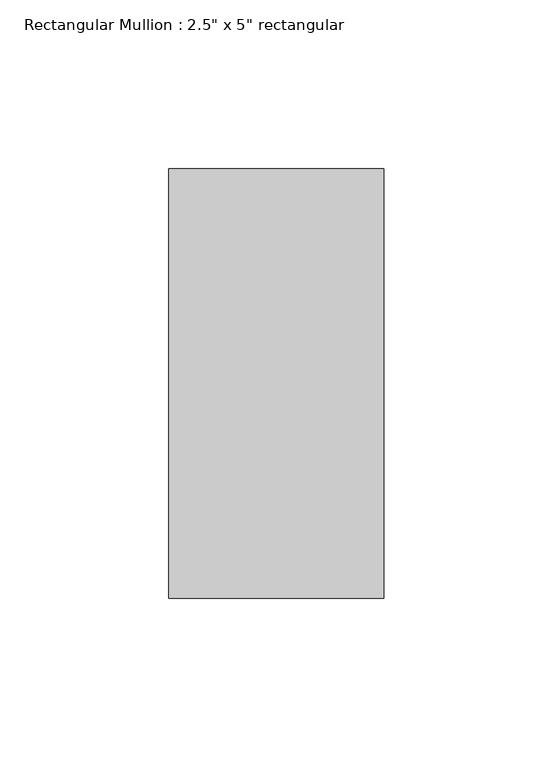
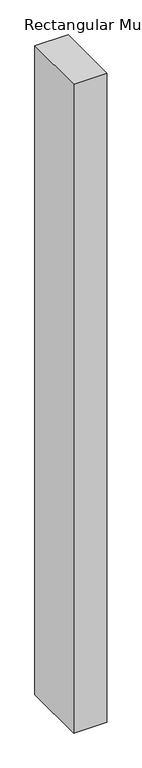
"""IFC4 building model written with IfcOpenShell, lengths in millimetres: member geometry."""

from ifc_helpers import new_model, si_unit, frame, origin, place, context, project, spatial, polyline, outline, extrude, source, transform, mapped, element, save


def member_fe35c162(model_context):
    return source(origin(), model_context, "Body", "SweptSolid", [
        extrude(outline(polyline([(0.0, 63.5), (0.0, -63.5), (-63.5, -63.5), (-63.5, 63.5), (0.0, 63.5)])), frame((0.0, 0.0, -1302.8083336), z_axis=(0.0, 0.0, 1.0), x_axis=(1.0, 0.0, 0.0)), (0.0, 0.0, 1.0), 1302.8083336),
    ])


if __name__ == "__main__":
    model = new_model("IFC4")
    model_context = context("Model", 3, world=origin())
    ifc_project = project(units=[si_unit("LENGTHUNIT", "METRE", prefix="MILLI")], contexts=[model_context])
    site = spatial("IfcSite", under=ifc_project)
    building = spatial("IfcBuilding", under=site)
    placement = place(None, origin())
    member_shape = member_fe35c162(model_context)
    element("IfcMember", 1, ObjectType="Rectangular Mullion : 2.5\" x 5\" rectangular", at=placement, inside=building, context=model_context, shape_type="MappedRepresentation", body=[
        mapped(member_shape, transform((0.0, 0.0, 0.0), x_axis=(1.0, 0.0, 0.0), y_axis=(0.0, 1.0, 0.0), z_axis=(0.0, 0.0, 1.0))),
    ])
    save(model, "model.ifc")

# Revit data of these elements
# Type "Rectangular Mullion : 2.5\" x 5\" rectangular"
#   built-in parameter 1007304 = 0.416667 (stored number, unit not read)
#   built-in parameter 1007301 = 0.104167 (stored number, unit not read)
#   built-in parameter 1007300 = 0.104167 (stored number, unit not read)
# Element 1 (IfcMember, "Rectangular Mullion : 2.5\" x 5\" rectangular")
#   Materials on its faces: "BLACK MATERIAL"
# Materials
#   "BLACK MATERIAL": class "Generic", colour RGB 120 120 120, transparency 0, Cost = 0
